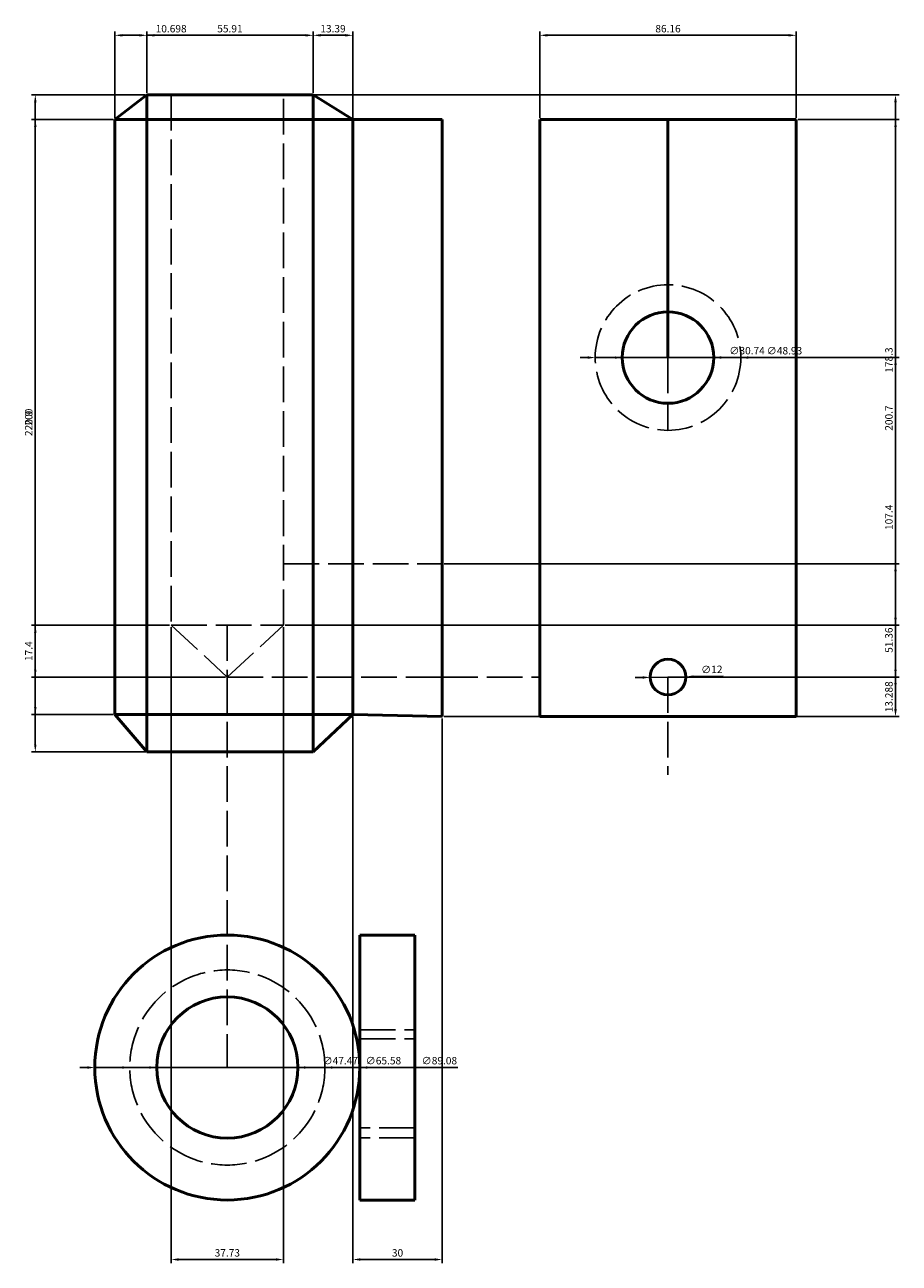
# Model space of a CAD drawing. Units: millimetres. Extents: x 921 to 2648, y 1390 to 2315.
# Tile 4 of 10: x 1465 to 1759, y 1494 to 1910. Entities that reach past the tile are written whole.
import ezdxf

# ---------------------------------------------------------------- set-up
doc = ezdxf.new("R2010")
doc.units = ezdxf.units.MM
doc.linetypes.add('ACAD_ISO02W100', pattern=[15, 12, -3])
for name, color, linetype, lineweight in [('M-DIMS', 2, 'Continuous', 25), ('M-HIDN', 4, 'ACAD_ISO02W100', 25), ('M-OUTL', 7, 'Continuous', 50)]:
    doc.layers.add(name, color=color, linetype=linetype, lineweight=lineweight)
doc.styles.get("Standard").update_dxf_attribs({"font": 'arial.ttf'})
doc.dimstyles.new('ISO-25', dxfattribs={"dimtxt": 2.5, "dimasz": 2.5, "dimexe": 1.25, "dimexo": 0.625, "dimtad": 1, "dimtxsty": 'Standard', "dimcen": 2.5, "dimadec": 0, "dimazin": 0, "dimtfac": 1, "dimtmove": 0, "dimatfit": 3, "dimfxl": 1, "dimarcsym": 0})

# ---------------------------------------------------------------- blocks, each defined once
blk = doc.blocks.new('*D29')
at = {"layer": 'Defpoints', "color": 0, "transparency": 16777216}
for p in [(1505.8, 1906.61), (1505.8, 1886.61), (1495.1, 1878.29)]:
    blk.add_point(p, dxfattribs=at)
at = {"layer": 'M-DIMS', "color": 0, "lineweight": -2, "transparency": 16777216}
for p, q in [((1495.1, 1878.91), (1495.1, 1907.86)), ((1505.8, 1887.23), (1505.8, 1907.86)), ((1497.6, 1906.61), (1503.3, 1906.61)), ((1505.8, 1906.61), (1519.7, 1906.61))]:
    blk.add_line(p, q, dxfattribs=at)
at = {"layer": 'M-DIMS', "color": 0, "transparency": 16777216}
for points in [[(1497.6, 1907.02), (1497.6, 1906.19), (1495.1, 1906.61)], [(1503.3, 1907.02), (1503.3, 1906.19), (1505.8, 1906.61)]]:
    blk.add_solid(points, dxfattribs=at)
at = {"layer": 'M-DIMS', "color": 0, "transparency": 16777216, "insert": (1514, 1908.51), "char_height": 2.5, "attachment_point": 5}
blk.add_mtext('10.698', dxfattribs=at)
blk = doc.blocks.new('*D30')
at = {"layer": 'Defpoints', "color": 0, "transparency": 16777216}
for p in [(1561.71, 1906.61), (1505.8, 1886.61), (1561.71, 1886.61)]:
    blk.add_point(p, dxfattribs=at)
at = {"layer": 'M-DIMS', "color": 0, "lineweight": -2, "transparency": 16777216}
for p, q in [((1505.8, 1887.23), (1505.8, 1907.86)), ((1561.71, 1887.23), (1561.71, 1907.86)), ((1508.3, 1906.61), (1559.21, 1906.61))]:
    blk.add_line(p, q, dxfattribs=at)
at = {"layer": 'M-DIMS', "color": 0, "transparency": 16777216}
for points in [[(1508.3, 1907.02), (1508.3, 1906.19), (1505.8, 1906.61)], [(1559.21, 1907.02), (1559.21, 1906.19), (1561.71, 1906.61)]]:
    blk.add_solid(points, dxfattribs=at)
at = {"layer": 'M-DIMS', "color": 0, "transparency": 16777216, "insert": (1533.76, 1908.51), "char_height": 2.5, "attachment_point": 5}
blk.add_mtext('55.91', dxfattribs=at)
blk = doc.blocks.new('*D31')
at = {"layer": 'Defpoints', "color": 0, "transparency": 16777216}
for p in [(1575.1, 1906.61), (1561.71, 1886.61), (1575.1, 1878.29)]:
    blk.add_point(p, dxfattribs=at)
at = {"layer": 'M-DIMS', "color": 0, "lineweight": -2, "transparency": 16777216}
for p, q in [((1561.71, 1887.23), (1561.71, 1907.86)), ((1575.1, 1878.91), (1575.1, 1907.86)), ((1564.21, 1906.61), (1572.6, 1906.61))]:
    blk.add_line(p, q, dxfattribs=at)
at = {"layer": 'M-DIMS', "color": 0, "transparency": 16777216}
for points in [[(1564.21, 1907.02), (1564.21, 1906.19), (1561.71, 1906.61)], [(1572.6, 1907.02), (1572.6, 1906.19), (1575.1, 1906.61)]]:
    blk.add_solid(points, dxfattribs=at)
at = {"layer": 'M-DIMS', "color": 0, "transparency": 16777216, "insert": (1568.41, 1908.51), "char_height": 2.5, "attachment_point": 5}
blk.add_mtext('13.39', dxfattribs=at)
blk = doc.blocks.new('*D32')
at = {"layer": 'Defpoints', "color": 0, "transparency": 16777216}
for p in [(1575.1, 1678.29), (1605.1, 1677.61), (1605.1, 1495.11)]:
    blk.add_point(p, dxfattribs=at)
at = {"layer": 'M-DIMS', "color": 0, "lineweight": -2, "transparency": 16777216}
for p, q in [((1575.1, 1677.66), (1575.1, 1493.86)), ((1605.1, 1676.98), (1605.1, 1493.86)), ((1577.6, 1495.11), (1602.6, 1495.11))]:
    blk.add_line(p, q, dxfattribs=at)
at = {"layer": 'M-DIMS', "color": 0, "transparency": 16777216}
for points in [[(1577.6, 1495.52), (1577.6, 1494.69), (1575.1, 1495.11)], [(1602.6, 1495.52), (1602.6, 1494.69), (1605.1, 1495.11)]]:
    blk.add_solid(points, dxfattribs=at)
at = {"layer": 'M-DIMS', "color": 0, "transparency": 16777216, "insert": (1590.1, 1497.01), "char_height": 2.5, "attachment_point": 5}
blk.add_mtext('30', dxfattribs=at)
blk = doc.blocks.new('*D33')
at = {"layer": 'Defpoints', "color": 0, "transparency": 16777216}
for p in [(1724.09, 1906.61), (1637.93, 1878.29), (1724.09, 1878.29)]:
    blk.add_point(p, dxfattribs=at)
at = {"layer": 'M-DIMS', "color": 0, "lineweight": -2, "transparency": 16777216}
for p, q in [((1637.93, 1878.91), (1637.93, 1907.86)), ((1724.09, 1878.91), (1724.09, 1907.86)), ((1640.43, 1906.61), (1721.59, 1906.61))]:
    blk.add_line(p, q, dxfattribs=at)
at = {"layer": 'M-DIMS', "color": 0, "transparency": 16777216}
for points in [[(1640.43, 1907.02), (1640.43, 1906.19), (1637.93, 1906.61)], [(1721.59, 1907.02), (1721.59, 1906.19), (1724.09, 1906.61)]]:
    blk.add_solid(points, dxfattribs=at)
at = {"layer": 'M-DIMS', "color": 0, "transparency": 16777216, "insert": (1681.01, 1908.51), "char_height": 2.5, "attachment_point": 5}
blk.add_mtext('86.16', dxfattribs=at)
blk = doc.blocks.new('*D74')
at = {"layer": 'Defpoints', "color": 0, "transparency": 16777216}
for p in [(1505.8, 1886.61), (1468.35, 1665.71), (1505.8, 1665.71)]:
    blk.add_point(p, dxfattribs=at)
at = {"layer": 'M-DIMS', "color": 0, "lineweight": -2, "transparency": 16777216}
for p, q in [((1505.18, 1886.61), (1467.1, 1886.61)), ((1468.35, 1884.11), (1468.35, 1668.21)), ((1505.18, 1665.71), (1467.1, 1665.71))]:
    blk.add_line(p, q, dxfattribs=at)
at = {"layer": 'M-DIMS', "color": 0, "transparency": 16777216}
for points in [[(1467.93, 1884.11), (1468.76, 1884.11), (1468.35, 1886.61)], [(1467.93, 1668.21), (1468.76, 1668.21), (1468.35, 1665.71)]]:
    blk.add_solid(points, dxfattribs=at)
at = {"layer": 'M-DIMS', "color": 0, "transparency": 16777216, "insert": (1466.45, 1776.16), "char_height": 2.5, "attachment_point": 5, "rotation": 90}
blk.add_mtext('220.9', dxfattribs=at)
blk = doc.blocks.new('*D75')
at = {"layer": 'Defpoints', "color": 0, "transparency": 16777216}
for p in [(1495.1, 1878.29), (1468.35, 1678.29), (1495.1, 1678.29)]:
    blk.add_point(p, dxfattribs=at)
at = {"layer": 'M-DIMS', "color": 0, "lineweight": -2, "transparency": 16777216}
for p, q in [((1494.48, 1878.29), (1467.1, 1878.29)), ((1468.35, 1875.79), (1468.35, 1680.79)), ((1494.48, 1678.29), (1467.1, 1678.29))]:
    blk.add_line(p, q, dxfattribs=at)
at = {"layer": 'M-DIMS', "color": 0, "transparency": 16777216}
for points in [[(1467.93, 1875.79), (1468.76, 1875.79), (1468.35, 1878.29)], [(1467.93, 1680.79), (1468.76, 1680.79), (1468.35, 1678.29)]]:
    blk.add_solid(points, dxfattribs=at)
at = {"layer": 'M-DIMS', "color": 0, "transparency": 16777216, "insert": (1466.45, 1778.29), "char_height": 2.5, "attachment_point": 5, "rotation": 90}
blk.add_mtext('200', dxfattribs=at)
blk = doc.blocks.new('*D76')
at = {"layer": 'Defpoints', "color": 0, "transparency": 16777216}
for p in [(1514.02, 1708.3), (1551.75, 1708.3), (1551.75, 1495.11)]:
    blk.add_point(p, dxfattribs=at)
at = {"layer": 'M-DIMS', "color": 0, "lineweight": -2, "transparency": 16777216}
for p, q in [((1514.02, 1707.67), (1514.02, 1493.86)), ((1551.75, 1707.67), (1551.75, 1493.86)), ((1516.52, 1495.11), (1549.25, 1495.11))]:
    blk.add_line(p, q, dxfattribs=at)
at = {"layer": 'M-DIMS', "color": 0, "transparency": 16777216}
for points in [[(1516.52, 1495.52), (1516.52, 1494.69), (1514.02, 1495.11)], [(1549.25, 1495.52), (1549.25, 1494.69), (1551.75, 1495.11)]]:
    blk.add_solid(points, dxfattribs=at)
at = {"layer": 'M-DIMS', "color": 0, "transparency": 16777216, "insert": (1532.89, 1497.01), "char_height": 2.5, "attachment_point": 5}
blk.add_mtext('37.73', dxfattribs=at)
blk = doc.blocks.new('*D77')
at = {"layer": 'Defpoints', "color": 0, "transparency": 16777216}
for p in [(1561.71, 1886.61), (1757.48, 1886.61), (1551.75, 1708.3)]:
    blk.add_point(p, dxfattribs=at)
at = {"layer": 'M-DIMS', "color": 0, "lineweight": -2, "transparency": 16777216}
for p, q in [((1562.34, 1886.61), (1758.73, 1886.61)), ((1757.48, 1710.8), (1757.48, 1884.11)), ((1552.38, 1708.3), (1758.73, 1708.3))]:
    blk.add_line(p, q, dxfattribs=at)
at = {"layer": 'M-DIMS', "color": 0, "transparency": 16777216}
for points in [[(1757.06, 1884.11), (1757.9, 1884.11), (1757.48, 1886.61)], [(1757.06, 1710.8), (1757.9, 1710.8), (1757.48, 1708.3)]]:
    blk.add_solid(points, dxfattribs=at)
at = {"layer": 'M-DIMS', "color": 0, "transparency": 16777216, "insert": (1755.58, 1797.45), "char_height": 2.5, "attachment_point": 5, "rotation": 90}
blk.add_mtext('178.3', dxfattribs=at)
blk = doc.blocks.new('*D78')
at = {"layer": 'Defpoints', "color": 0, "transparency": 16777216}
for p in [(1514.02, 1708.3), (1468.35, 1690.9), (1532.89, 1690.9)]:
    blk.add_point(p, dxfattribs=at)
at = {"layer": 'M-DIMS', "color": 0, "lineweight": -2, "transparency": 16777216}
for p, q in [((1513.4, 1708.3), (1467.1, 1708.3)), ((1468.35, 1705.8), (1468.35, 1693.4)), ((1532.26, 1690.9), (1467.1, 1690.9))]:
    blk.add_line(p, q, dxfattribs=at)
at = {"layer": 'M-DIMS', "color": 0, "transparency": 16777216}
for points in [[(1467.93, 1705.8), (1468.76, 1705.8), (1468.35, 1708.3)], [(1467.93, 1693.4), (1468.76, 1693.4), (1468.35, 1690.9)]]:
    blk.add_solid(points, dxfattribs=at)
at = {"layer": 'M-DIMS', "color": 0, "transparency": 16777216, "insert": (1466.47, 1699.6), "char_height": 2.5, "attachment_point": 5, "rotation": 90}
blk.add_mtext('17.4', dxfattribs=at)
blk = doc.blocks.new('*D79')
at = {"layer": 'Defpoints', "color": 0, "transparency": 16777216}
for p in [(1605.1, 1728.97), (1605.1, 1677.61), (1757.48, 1677.61)]:
    blk.add_point(p, dxfattribs=at)
at = {"layer": 'M-DIMS', "color": 0, "lineweight": -2, "transparency": 16777216}
for p, q in [((1605.73, 1728.97), (1758.73, 1728.97)), ((1757.48, 1726.47), (1757.48, 1680.11)), ((1605.73, 1677.61), (1758.73, 1677.61))]:
    blk.add_line(p, q, dxfattribs=at)
at = {"layer": 'M-DIMS', "color": 0, "transparency": 16777216}
for points in [[(1757.06, 1726.47), (1757.9, 1726.47), (1757.48, 1728.97)], [(1757.06, 1680.11), (1757.9, 1680.11), (1757.48, 1677.61)]]:
    blk.add_solid(points, dxfattribs=at)
at = {"layer": 'M-DIMS', "color": 0, "transparency": 16777216, "insert": (1755.58, 1703.29), "char_height": 2.5, "attachment_point": 5, "rotation": 90}
blk.add_mtext('51.36', dxfattribs=at)
blk = doc.blocks.new('*D80')
at = {"layer": 'Defpoints', "color": 0, "transparency": 16777216}
for p in [(1724.09, 1878.29), (1724.09, 1677.61), (1757.48, 1677.61)]:
    blk.add_point(p, dxfattribs=at)
at = {"layer": 'M-DIMS', "color": 0, "lineweight": -2, "transparency": 16777216}
for p, q in [((1724.71, 1878.29), (1758.73, 1878.29)), ((1757.48, 1875.79), (1757.48, 1680.11)), ((1724.71, 1677.61), (1758.73, 1677.61))]:
    blk.add_line(p, q, dxfattribs=at)
at = {"layer": 'M-DIMS', "color": 0, "transparency": 16777216}
for points in [[(1757.06, 1875.79), (1757.9, 1875.79), (1757.48, 1878.29)], [(1757.06, 1680.11), (1757.9, 1680.11), (1757.48, 1677.61)]]:
    blk.add_solid(points, dxfattribs=at)
at = {"layer": 'M-DIMS', "color": 0, "transparency": 16777216, "insert": (1755.58, 1777.95), "char_height": 2.5, "attachment_point": 5, "rotation": 90}
blk.add_mtext('200.7', dxfattribs=at)
blk = doc.blocks.new('*D81')
at = {"layer": 'Defpoints', "color": 0, "transparency": 16777216}
for p in [(1681.01, 1690.9), (1757.48, 1690.9), (1724.09, 1677.61)]:
    blk.add_point(p, dxfattribs=at)
at = {"layer": 'M-DIMS', "color": 0, "lineweight": -2, "transparency": 16777216}
for p, q in [((1681.63, 1690.9), (1758.73, 1690.9)), ((1757.48, 1680.11), (1757.48, 1688.4)), ((1724.71, 1677.61), (1758.73, 1677.61))]:
    blk.add_line(p, q, dxfattribs=at)
at = {"layer": 'M-DIMS', "color": 0, "transparency": 16777216}
for points in [[(1757.06, 1688.4), (1757.9, 1688.4), (1757.48, 1690.9)], [(1757.06, 1680.11), (1757.9, 1680.11), (1757.48, 1677.61)]]:
    blk.add_solid(points, dxfattribs=at)
at = {"layer": 'M-DIMS', "color": 0, "transparency": 16777216, "insert": (1755.58, 1684.25), "char_height": 2.5, "attachment_point": 5, "rotation": 90}
blk.add_mtext('13.288', dxfattribs=at)
blk = doc.blocks.new('*D82')
at = {"layer": 'Defpoints', "color": 0, "transparency": 16777216}
for p in [(1681.01, 1798.29), (1757.48, 1798.29), (1681.01, 1690.9)]:
    blk.add_point(p, dxfattribs=at)
at = {"layer": 'M-DIMS', "color": 0, "lineweight": -2, "transparency": 16777216}
for p, q in [((1681.63, 1798.29), (1758.73, 1798.29)), ((1757.48, 1693.4), (1757.48, 1795.79)), ((1681.63, 1690.9), (1758.73, 1690.9))]:
    blk.add_line(p, q, dxfattribs=at)
at = {"layer": 'M-DIMS', "color": 0, "transparency": 16777216}
for points in [[(1757.06, 1795.79), (1757.9, 1795.79), (1757.48, 1798.29)], [(1757.06, 1693.4), (1757.9, 1693.4), (1757.48, 1690.9)]]:
    blk.add_solid(points, dxfattribs=at)
at = {"layer": 'M-DIMS', "color": 0, "transparency": 16777216, "insert": (1755.58, 1744.59), "char_height": 2.5, "attachment_point": 5, "rotation": 90}
blk.add_mtext('107.4', dxfattribs=at)
blk = doc.blocks.new('*D114')
at = {"layer": 'Defpoints', "color": 0, "transparency": 16777216}
for p in [(1488.35, 1559.65), (1577.43, 1559.65)]:
    blk.add_point(p, dxfattribs=at)
at = {"layer": 'M-DIMS', "color": 0, "lineweight": -2, "transparency": 16777216}
for p, q in [((1485.85, 1559.65), (1483.35, 1559.65)), ((1488.35, 1559.65), (1577.43, 1559.65)), ((1610.36, 1559.65), (1579.93, 1559.65))]:
    blk.add_line(p, q, dxfattribs=at)
at = {"layer": 'M-DIMS', "color": 0, "transparency": 16777216}
for points in [[(1485.85, 1560.06), (1485.85, 1559.23), (1488.35, 1559.65)], [(1579.93, 1560.06), (1579.93, 1559.23), (1577.43, 1559.65)]]:
    blk.add_solid(points, dxfattribs=at)
at = {"layer": 'M-DIMS', "color": 0, "transparency": 16777216, "insert": (1604.15, 1561.62), "char_height": 2.5, "attachment_point": 5, "rotation": 359.9994}
blk.add_mtext('∅89.08', dxfattribs=at)
blk = doc.blocks.new('*D115')
at = {"layer": 'Defpoints', "color": 0, "transparency": 16777216}
for p in [(1500.1, 1559.65), (1565.68, 1559.65)]:
    blk.add_point(p, dxfattribs=at)
at = {"layer": 'M-DIMS', "color": 0, "lineweight": -2, "transparency": 16777216}
for p, q in [((1497.6, 1559.65), (1495.1, 1559.65)), ((1500.1, 1559.65), (1565.68, 1559.65)), ((1591.56, 1559.65), (1568.18, 1559.65))]:
    blk.add_line(p, q, dxfattribs=at)
at = {"layer": 'M-DIMS', "color": 0, "transparency": 16777216}
for points in [[(1497.6, 1560.06), (1497.6, 1559.23), (1500.1, 1559.65)], [(1568.18, 1560.06), (1568.18, 1559.23), (1565.68, 1559.65)]]:
    blk.add_solid(points, dxfattribs=at)
at = {"layer": 'M-DIMS', "color": 0, "transparency": 16777216, "insert": (1585.35, 1561.62), "char_height": 2.5, "attachment_point": 5, "rotation": 359.9991}
blk.add_mtext('∅65.58', dxfattribs=at)
blk = doc.blocks.new('*D116')
at = {"layer": 'Defpoints', "color": 0, "transparency": 16777216}
for p in [(1509.15, 1559.65), (1556.62, 1559.65)]:
    blk.add_point(p, dxfattribs=at)
at = {"layer": 'M-DIMS', "color": 0, "lineweight": -2, "transparency": 16777216}
for p, q in [((1506.65, 1559.65), (1504.15, 1559.65)), ((1509.15, 1559.65), (1556.62, 1559.65)), ((1577.07, 1559.65), (1559.12, 1559.65))]:
    blk.add_line(p, q, dxfattribs=at)
at = {"layer": 'M-DIMS', "color": 0, "transparency": 16777216}
for points in [[(1506.65, 1560.06), (1506.65, 1559.23), (1509.15, 1559.65)], [(1559.12, 1560.06), (1559.12, 1559.23), (1556.62, 1559.65)]]:
    blk.add_solid(points, dxfattribs=at)
at = {"layer": 'M-DIMS', "color": 0, "transparency": 16777216, "insert": (1570.86, 1561.62), "char_height": 2.5, "attachment_point": 5, "rotation": 359.9988}
blk.add_mtext('∅47.47', dxfattribs=at)
blk = doc.blocks.new('*D117')
at = {"layer": 'Defpoints', "color": 0, "transparency": 16777216}
for p in [(1656.54, 1798.29), (1705.47, 1798.29)]:
    blk.add_point(p, dxfattribs=at)
at = {"layer": 'M-DIMS', "color": 0, "lineweight": -2, "transparency": 16777216}
for p, q in [((1654.04, 1798.29), (1651.54, 1798.29)), ((1656.54, 1798.29), (1705.47, 1798.29)), ((1726.36, 1798.29), (1707.97, 1798.29))]:
    blk.add_line(p, q, dxfattribs=at)
at = {"layer": 'M-DIMS', "color": 0, "transparency": 16777216}
for points in [[(1654.04, 1798.71), (1654.04, 1797.87), (1656.54, 1798.29)], [(1707.97, 1798.71), (1707.97, 1797.87), (1705.47, 1798.29)]]:
    blk.add_solid(points, dxfattribs=at)
at = {"layer": 'M-DIMS', "color": 0, "transparency": 16777216, "insert": (1720.15, 1800.26), "char_height": 2.5, "attachment_point": 5, "rotation": 0.0004}
blk.add_mtext('∅48.93', dxfattribs=at)
blk = doc.blocks.new('*D136')
at = {"layer": 'Defpoints', "color": 0, "transparency": 16777216}
for p in [(1665.64, 1798.28), (1696.38, 1798.3)]:
    blk.add_point(p, dxfattribs=at)
at = {"layer": 'M-DIMS', "color": 0, "lineweight": -2, "transparency": 16777216}
for p, q in [((1663.14, 1798.28), (1660.64, 1798.28)), ((1665.64, 1798.28), (1696.38, 1798.3)), ((1713.77, 1798.31), (1698.88, 1798.3))]:
    blk.add_line(p, q, dxfattribs=at)
at = {"layer": 'M-DIMS', "color": 0, "transparency": 16777216}
for points in [[(1663.14, 1798.69), (1663.14, 1797.86), (1665.64, 1798.28)], [(1698.88, 1798.72), (1698.88, 1797.89), (1696.38, 1798.3)]]:
    blk.add_solid(points, dxfattribs=at)
at = {"layer": 'M-DIMS', "color": 0, "transparency": 16777216, "insert": (1707.58, 1800.28), "char_height": 2.5, "attachment_point": 5, "rotation": 0.0381}
blk.add_mtext('∅30.74', dxfattribs=at)
blk = doc.blocks.new('*D137')
at = {"layer": 'Defpoints', "color": 0, "transparency": 16777216}
for p in [(1675.01, 1690.79), (1687.01, 1691)]:
    blk.add_point(p, dxfattribs=at)
at = {"layer": 'M-DIMS', "color": 0, "lineweight": -2, "transparency": 16777216}
for p, q in [((1672.51, 1690.75), (1670.01, 1690.7)), ((1675.01, 1690.79), (1687.01, 1691)), ((1699.53, 1691.22), (1689.51, 1691.04))]:
    blk.add_line(p, q, dxfattribs=at)
at = {"layer": 'M-DIMS', "color": 0, "transparency": 16777216}
for points in [[(1672.5, 1691.16), (1672.52, 1690.33), (1675.01, 1690.79)], [(1689.5, 1691.46), (1689.51, 1690.63), (1687.01, 1691)]]:
    blk.add_solid(points, dxfattribs=at)
at = {"layer": 'M-DIMS', "color": 0, "transparency": 16777216, "insert": (1695.73, 1693.12), "char_height": 2.5, "attachment_point": 5, "rotation": 0.9969}
blk.add_mtext('∅12', dxfattribs=at)

msp = doc.modelspace()

# ---------------------------------------------------------------- linework, layer by layer
at = {"layer": 'M-HIDN'}
for p, q in [((1514.0233, 1886.6083), (1514.0233, 1708.297)), ((1551.7502, 1708.297), (1551.7502, 1886.6083)), ((1681.0074, 1798.2898), (1681.0074, 1773.8235)), ((1551.7502, 1728.9711), (1605.1044, 1728.9711)), ((1514.0233, 1708.297), (1551.7502, 1708.297)), ((1514.0233, 1708.297), (1532.8867, 1690.8957)), ((1532.8867, 1708.297), (1532.8867, 1690.8957)), ((1532.8867, 1690.8957), (1551.7502, 1708.297)), ((1532.8867, 1690.8957), (1605.1044, 1690.8957)), ((1532.8867, 1690.8957), (1532.8867, 1559.6465)), ((1605.1044, 1690.8957), (1637.9267, 1690.8957)), ((1681.0074, 1690.8957), (1737.4801, 1690.8957)), ((1681.0074, 1690.8957), (1681.0074, 1658.041)), ((1577.4268, 1572.3434), (1595.9129, 1572.3434)), ((1577.4268, 1569.3397), (1595.9129, 1569.3397)), ((1595.9129, 1539.3397), (1577.4268, 1539.3397)), ((1595.9129, 1536.0591), (1577.4268, 1536.0591))]:
    msp.add_line(p, q, dxfattribs=at)
for centre, radius in [((1681.0074, 1798.2898), 24.4663), ((1532.8867, 1559.6465), 32.791)]:
    msp.add_circle(centre, radius, dxfattribs=at)
at = {"layer": 'M-OUTL'}
for p, q in [((1505.8021, 1886.6083), (1495.1044, 1878.2898)), ((1505.8021, 1886.6083), (1561.7149, 1886.6083)), ((1505.8021, 1886.6083), (1505.8021, 1665.7078)), ((1561.7149, 1886.6083), (1561.7149, 1665.7078)), ((1561.7149, 1886.6083), (1575.1044, 1878.2898)), ((1495.1044, 1878.2898), (1575.1044, 1878.2898)), ((1495.1044, 1678.2898), (1495.1044, 1878.2898)), ((1575.1044, 1878.2898), (1575.1044, 1678.2898)), ((1575.1044, 1878.2898), (1605.1044, 1878.2898)), ((1605.1044, 1878.2898), (1605.1044, 1677.6078)), ((1637.9267, 1878.2898), (1637.9267, 1677.6078)), ((1637.9267, 1878.2898), (1724.0881, 1878.2898)), ((1681.0074, 1878.2898), (1681.0074, 1798.2898)), ((1724.0881, 1878.2898), (1724.0881, 1677.6078)), ((1575.1044, 1678.2898), (1495.1044, 1678.2898)), ((1505.8021, 1665.7078), (1495.1044, 1678.2898)), ((1575.1044, 1678.2898), (1561.7149, 1665.7078)), ((1605.1044, 1677.6078), (1575.1044, 1678.2898)), ((1637.9267, 1677.6078), (1724.0881, 1677.6078)), ((1561.7149, 1665.7078), (1505.8021, 1665.7078)), ((1577.4268, 1559.6465), (1577.4268, 1604.1866)), ((1577.4268, 1604.1866), (1595.9129, 1604.1866)), ((1595.9129, 1604.1866), (1595.9129, 1515.1064)), ((1577.4268, 1559.6465), (1577.4268, 1515.1064)), ((1577.4268, 1515.1064), (1595.9129, 1515.1064))]:
    msp.add_line(p, q, dxfattribs=at)
for centre, radius in [((1681.0074, 1798.2898), 15.3711), ((1681.0074, 1690.8957), 6), ((1532.8867, 1559.6465), 44.5401), ((1532.8867, 1559.6465), 44.5401), ((1532.8867, 1559.6465), 23.7359)]:
    msp.add_circle(centre, radius, dxfattribs=at)

# ---------------------------------------------------------------- dimensions: what is measured, and where the dimension line sits
at = {"layer": 'M-DIMS'}
for base, p1, p2, override, picture, middle in [((1505.8021, 1906.6083), (1495.1044, 1878.2898), (1505.8021, 1886.6083), {"dimdec": 3, "dimlfac": 1, "dimrnd": 0, "dimzin": 0, "dimdsep": 46, "dimlunit": 2}, '*D29', (1514.0013, 1908.5097)), ((1561.7149, 1906.6083), (1505.8021, 1886.6083), (1561.7149, 1886.6083), {"dimdec": 2, "dimlfac": 1, "dimrnd": 0, "dimzin": 0, "dimdsep": 46, "dimlunit": 2}, '*D30', (1533.7585, 1908.5097)), ((1575.1044, 1906.6083), (1561.7149, 1886.6083), (1575.1044, 1878.2898), {"dimdec": 2, "dimlfac": 1, "dimrnd": 0, "dimzin": 0, "dimdsep": 46, "dimlunit": 2}, '*D31', (1568.4097, 1908.5106)), ((1724.0881, 1906.6083), (1637.9267, 1878.2898), (1724.0881, 1878.2898), {"dimdec": 2, "dimlfac": 1, "dimrnd": 0, "dimzin": 0, "dimdsep": 46, "dimlunit": 2}, '*D33', (1681.0074, 1908.5097)), ((1551.7502, 1495.1064), (1514.0233, 1708.297), (1551.7502, 1708.297), {"dimdec": 2, "dimlfac": 1, "dimrnd": 0, "dimzin": 0, "dimdsep": 46, "dimlunit": 2}, '*D76', (1532.8867, 1497.0087)), ((1605.1044, 1495.1064), (1575.1044, 1678.2898), (1605.1044, 1677.6078), {"dimdec": 0, "dimlfac": 1, "dimrnd": 0, "dimzin": 0, "dimdsep": 46, "dimlunit": 2}, '*D32', (1590.1044, 1497.0087))]:
    dim = msp.add_linear_dim(base=base, p1=p1, p2=p2, dimstyle='ISO-25', override=override, dxfattribs=at)
    dim.commit()
    dim.dimension.update_dxf_attribs({"geometry": picture, "text_midpoint": middle})
for base, p1, p2, override, picture, middle in [((1468.3467, 1665.7078), (1505.8021, 1886.6083), (1505.8021, 1665.7078), {"dimdec": 1, "dimlfac": 1, "dimrnd": 0, "dimzin": 0, "dimdsep": 46, "dimlunit": 2}, '*D74', (1466.4452, 1776.158)), ((1757.4801, 1886.6083), (1551.7502, 1708.297), (1561.7149, 1886.6083), {"dimdec": 1, "dimlfac": 1, "dimrnd": 0, "dimzin": 0, "dimdsep": 46, "dimlunit": 2}, '*D77', (1755.5778, 1797.4526)), ((1468.3467, 1678.2898), (1495.1044, 1878.2898), (1495.1044, 1678.2898), {"dimdec": 0, "dimlfac": 1, "dimrnd": 0, "dimzin": 0, "dimdsep": 46, "dimlunit": 2}, '*D75', (1466.4452, 1778.2898)), ((1757.4801, 1677.6078), (1724.0881, 1878.2898), (1724.0881, 1677.6078), {"dimdec": 1, "dimlfac": 1, "dimrnd": 0, "dimzin": 0, "dimdsep": 46, "dimlunit": 2}, '*D80', (1755.5787, 1777.9488)), ((1757.4801, 1798.2898), (1681.0074, 1690.8957), (1681.0074, 1798.2898), {"dimdec": 1, "dimlfac": 1, "dimrnd": 0, "dimzin": 0, "dimdsep": 46, "dimlunit": 2}, '*D82', (1755.5787, 1744.5928)), ((1757.4801, 1677.6078), (1605.1044, 1728.9711), (1605.1044, 1677.6078), {"dimdec": 2, "dimlfac": 1, "dimrnd": 0, "dimzin": 0, "dimdsep": 46, "dimlunit": 2}, '*D79', (1755.5778, 1703.2895)), ((1468.3467, 1690.8957), (1514.0233, 1708.297), (1532.8867, 1690.8957), {"dimdec": 1, "dimlfac": 1, "dimrnd": 0, "dimzin": 0, "dimdsep": 46, "dimlunit": 2}, '*D78', (1466.4666, 1699.5963)), ((1757.4801, 1690.8957), (1724.0881, 1677.6078), (1681.0074, 1690.8957), {"dimdec": 3, "dimlfac": 1, "dimrnd": 0, "dimzin": 0, "dimdsep": 46, "dimlunit": 2}, '*D81', (1755.5778, 1684.2518))]:
    dim = msp.add_linear_dim(base=base, p1=p1, p2=p2, angle=90, dimstyle='ISO-25', override=override, dxfattribs=at)
    dim.commit()
    dim.dimension.update_dxf_attribs({"geometry": picture, "text_midpoint": middle})
for p1, p2, override, picture, middle in [((1656.5411, 1798.2897), (1705.4737, 1798.29), {"dimdec": 2, "dimlfac": 1, "dimrnd": 0, "dimzin": 0, "dimdsep": 46, "dimlunit": 2}, '*D117', (1720.1535, 1798.2901)), ((1665.6363, 1798.2796), (1696.3784, 1798.3001), {"dimdec": 2, "dimlfac": 1, "dimrnd": 0, "dimzin": 0, "dimdsep": 46, "dimlunit": 2}, '*D136', (1707.5764, 1798.3075)), ((1675.0083, 1690.7913), (1687.0065, 1691.0001), {"dimdec": 0, "dimlfac": 1, "dimrnd": 0, "dimzin": 0, "dimdsep": 46, "dimlunit": 2}, '*D137', (1695.7679, 1691.1526)), ((1488.3467, 1559.647), (1577.4268, 1559.646), {"dimdec": 2, "dimlfac": 1, "dimrnd": 0, "dimzin": 0, "dimdsep": 46, "dimlunit": 2}, '*D114', (1604.1508, 1559.6457)), ((1500.0957, 1559.647), (1565.6777, 1559.646), {"dimdec": 2, "dimlfac": 1, "dimrnd": 0, "dimzin": 0, "dimdsep": 46, "dimlunit": 2}, '*D115', (1585.3523, 1559.6457)), ((1509.1509, 1559.647), (1556.6226, 1559.646), {"dimdec": 2, "dimlfac": 1, "dimrnd": 0, "dimzin": 0, "dimdsep": 46, "dimlunit": 2}, '*D116', (1570.8641, 1559.6457))]:
    dim = msp.add_diameter_dim_2p(p1=p1, p2=p2, dimstyle='ISO-25', override=override, dxfattribs=at)
    dim.commit()
    dim.dimension.update_dxf_attribs({"geometry": picture, "text_midpoint": middle, "dimtype": 163})

doc.saveas('drawing.dxf')
